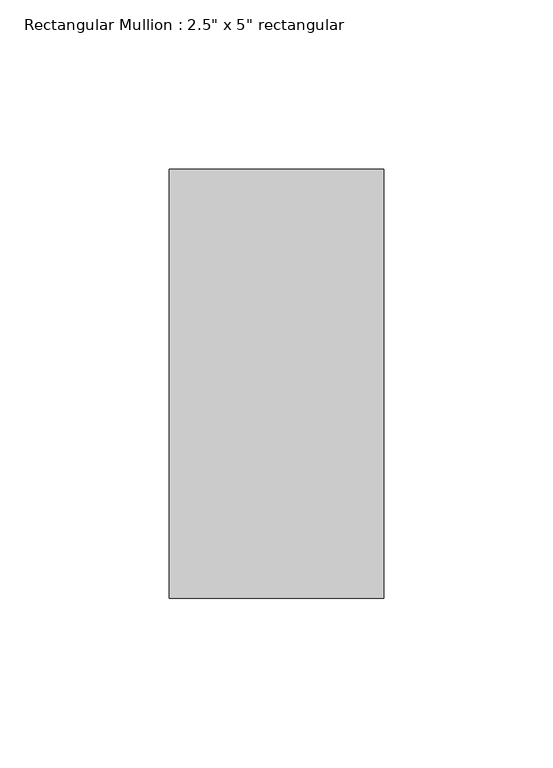
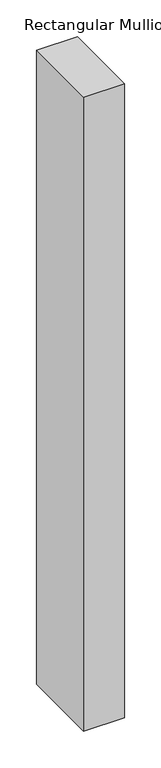
"""IFC4 building model written with IfcOpenShell, lengths in millimetres: member geometry."""

from ifc_helpers import new_model, si_unit, frame, origin, place, context, project, spatial, polyline, outline, extrude, source, transform, mapped, element, save


def member_2a6e7b3e(model_context):
    return source(origin(), model_context, "Body", "SweptSolid", [
        extrude(outline(polyline([(0.0, 63.5), (0.0, -63.5), (-63.5, -63.5), (-63.5, 63.5), (0.0, 63.5)])), frame((0.0, 0.0, -1047.3490947), z_axis=(0.0, 0.0, 1.0), x_axis=(1.0, 0.0, 0.0)), (0.0, 0.0, 1.0), 1047.3490947),
    ])


if __name__ == "__main__":
    model = new_model("IFC4")
    model_context = context("Model", 3, world=origin())
    ifc_project = project(units=[si_unit("LENGTHUNIT", "METRE", prefix="MILLI")], contexts=[model_context])
    site = spatial("IfcSite", under=ifc_project)
    building = spatial("IfcBuilding", under=site)
    placement = place(None, origin())
    member_shape = member_2a6e7b3e(model_context)
    element("IfcMember", 1, ObjectType="Rectangular Mullion : 2.5\" x 5\" rectangular", at=placement, inside=building, context=model_context, shape_type="MappedRepresentation", body=[
        mapped(member_shape, transform((0.0, 0.0, 0.0), x_axis=(1.0, 0.0, 0.0), y_axis=(0.0, 1.0, 0.0), z_axis=(0.0, 0.0, 1.0))),
    ])
    save(model, "model.ifc")

# Revit data of these elements
# Type "Rectangular Mullion : 2.5\" x 5\" rectangular"
#   built-in parameter 1007304 = 0.416667 (stored number, unit not read)
#   built-in parameter 1007301 = 0.104167 (stored number, unit not read)
#   built-in parameter 1007300 = 0.104167 (stored number, unit not read)
# Element 1 (IfcMember, "Rectangular Mullion : 2.5\" x 5\" rectangular")
#   Materials on its faces: "Aluminum"
# Materials
#   "Aluminum": class "Metal", colour RGB 247 247 247, transparency 0, Description = "Aluminum 6061", Cost = 0
